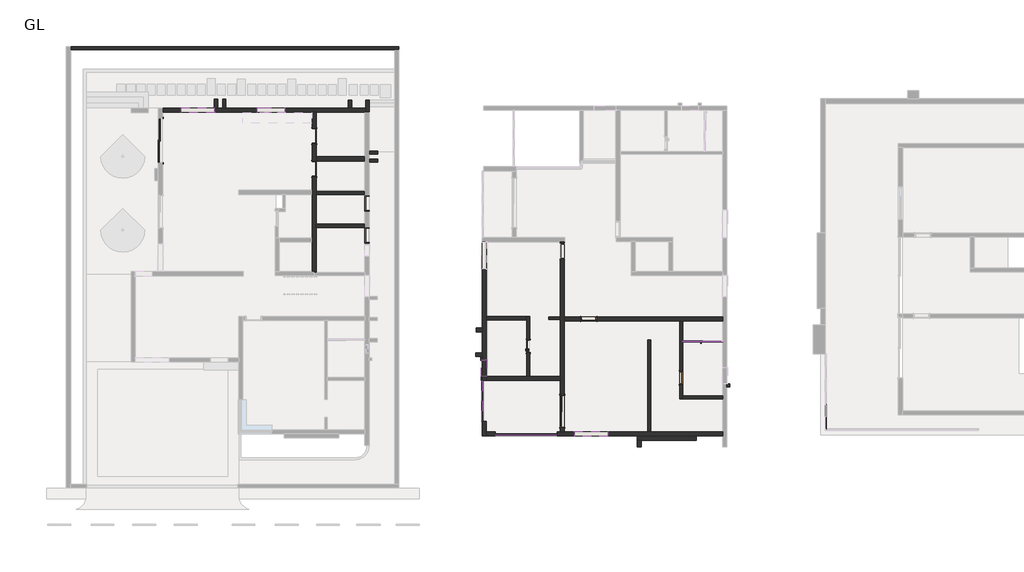
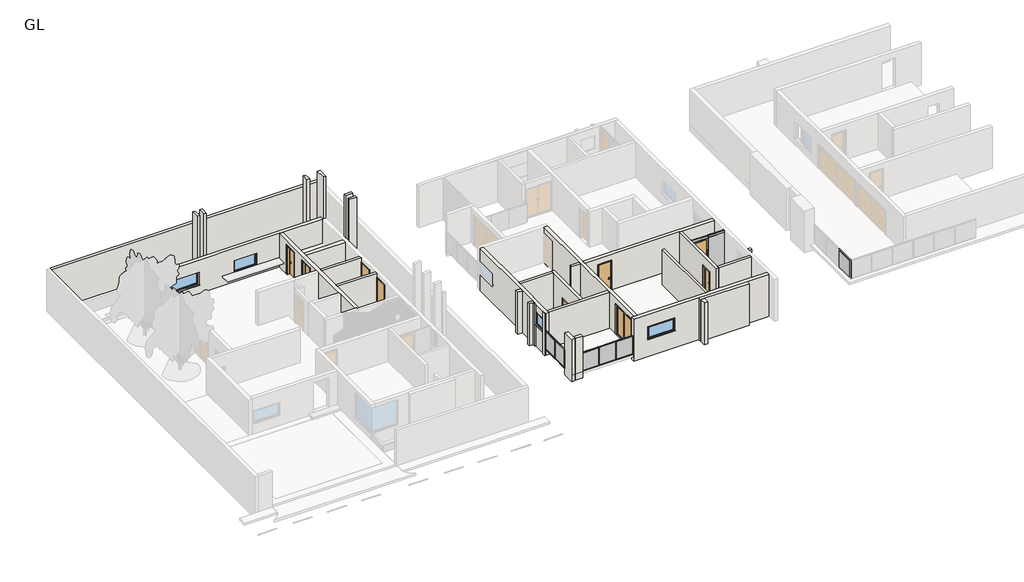
# One storey, part 2 of 6: 32 walls, 26 members, 10 doors, 9 plates, 4 windows.
"""IFC4 building model written with IfcOpenShell, lengths in millimetres."""

from ifc_helpers import new_model, si_unit, origin, origin_with_axes, place, context, project, spatial, polyline, outline, extrude, faceted_brep, transform, mapped, element, save
from components import door_510b0506, door_8_4088deed, door_61435f0d, door_b7cddb0a, doors_intsgl_2_5_55235da4, doors_intsgl_2_5_ea0f4f48, doors_sgl_glass_1_glass_panel_12mm_thickness_f5485519, rectangular_mullion_30mm_square_7ad516a4, rectangular_mullion_30mm_square_4b249e81, rectangular_mullion_30mm_square_698bad25, rectangular_mullion_30mm_square_c90eb03c, rectangular_mullion_30mm_square_82a776c0, rectangular_mullion_30mm_square_9325025b, rectangular_mullion_30mm_square_e994106c, rectangular_mullion_30mm_square_b4ecd99e, rectangular_mullion_30mm_square_28ebc8b3, rectangular_mullion_30mm_square_04db908b, rectangular_mullion_30mm_square_ca2d7245, system_panel_glazed_e1dbe616, system_panel_glazed_3d395eef, system_panel_glazed_b6747f4f, system_panel_glazed_7d86dfa2, system_panel_glazed_82719d7e, windows_sgl_plain_3_28d0678b, windows_sgl_plain_5_c2f68037, windows_sgl_plain_6_060cc830

model = new_model("IFC4")

# Units and contexts
model_context = context("Model", 3, world=origin())
ifc_project = project(units=[si_unit("LENGTHUNIT", "METRE", prefix="MILLI")], contexts=[model_context])

# Site, building, storey
site = spatial("IfcSite", under=ifc_project)
building = spatial("IfcBuilding", under=site)
storey = spatial("IfcBuildingStorey", under=building, Name="GL", Elevation=0.0)

# Doors
placement = place(None, origin())
door_shape = door_510b0506(model_context)
element("IfcDoor", 1, ObjectType="5'10\"", at=placement, inside=storey, context=model_context, shape_type="MappedRepresentation", body=[
    mapped(door_shape, transform((-24575.6081987, 10334.3302878, 449.9570313), x_axis=(0.0, 1.0, 0.0), y_axis=(-1.0, 0.0, 0.0), z_axis=(0.0, 0.0, 1.0))),
])
door_8_shape = door_8_4088deed(model_context)
element("IfcDoor", 2, ObjectType="8'", at=placement, inside=storey, context=model_context, shape_type="MappedRepresentation", body=[
    mapped(door_8_shape, transform((-46875.1786333, 25369.1148243, 449.9570313), x_axis=(0.0, 1.0, 0.0), y_axis=(-1.0, 0.0, 0.0), z_axis=(0.0, 0.0, 1.0))),
])
door_2_shape = door_61435f0d(model_context)
element("IfcDoor", 3, ObjectType="Doors_IntSgl : 2'11\"", at=placement, inside=storey, context=model_context, shape_type="MappedRepresentation", body=[
    mapped(door_2_shape, transform((-35537.04796, 20098.7041063, 589.9546875), x_axis=(0.0, 1.0, 0.0), y_axis=(-1.0, 0.0, 0.0), z_axis=(0.0, 0.0, 1.0))),
])
element("IfcDoor", 4, ObjectType="Doors_IntSgl : 2'11\"", at=placement, inside=storey, context=model_context, shape_type="MappedRepresentation", body=[
    mapped(door_2_shape, transform((-38458.04796, 25623.2041063, 589.9546875), x_axis=(0.0, -1.0, 0.0), y_axis=(1.0, 0.0, 0.0), z_axis=(0.0, 0.0, 1.0))),
])
element("IfcDoor", 5, ObjectType="Doors_IntSgl : 2'11\"", at=placement, inside=storey, context=model_context, shape_type="MappedRepresentation", body=[
    mapped(door_2_shape, transform((-35537.04796, 21876.7041063, 589.9546875), x_axis=(0.0, 1.0, 0.0), y_axis=(-1.0, 0.0, 0.0), z_axis=(0.0, 0.0, 1.0))),
])
element("IfcDoor", 6, ObjectType="Doors_IntSgl : 2'11\"", at=placement, inside=storey, context=model_context, shape_type="MappedRepresentation", body=[
    mapped(door_2_shape, transform((-23229.4081987, 15463.5822323, 449.9429688), x_axis=(-1.0, 0.0, 0.0), y_axis=(0.0, -1.0, 0.0), z_axis=(0.0, 0.0, 1.0))),
])
door_3_shape = door_b7cddb0a(model_context)
element("IfcDoor", 7, ObjectType="Doors_IntSgl : 2'11\"", at=placement, inside=storey, context=model_context, shape_type="MappedRepresentation", body=[
    mapped(door_3_shape, transform((-38458.04796, 23794.4041063, 589.9546875), x_axis=(0.0, 1.0, 0.0), y_axis=(-1.0, 0.0, 0.0), z_axis=(0.0, 0.0, 1.0))),
])
doors_intsgl_2_5_shape = doors_intsgl_2_5_55235da4(model_context)
element("IfcDoor", 8, ObjectType="Doors_IntSgl : 2.5'", at=placement, inside=storey, context=model_context, shape_type="MappedRepresentation", body=[
    mapped(doors_intsgl_2_5_shape, transform((-18095.11552, 12186.9822323, 449.9570313), x_axis=(0.0, 1.0, 0.0), y_axis=(-1.0, 0.0, 0.0), z_axis=(0.0, 0.0, 1.0))),
])
doors_intsgl_2_5_2_shape = doors_intsgl_2_5_ea0f4f48(model_context)
element("IfcDoor", 9, ObjectType="Doors_IntSgl : 2.5'", at=placement, inside=storey, context=model_context, shape_type="MappedRepresentation", body=[
    mapped(doors_intsgl_2_5_2_shape, transform((-26580.8290616, 13941.6413647, 0.0), x_axis=(0.0, 1.0, 0.0), y_axis=(-1.0, 0.0, 0.0), z_axis=(0.0, 0.0, 1.0))),
])
doors_sgl_glass_1_glass_panel_12mm_thickness_shape = doors_sgl_glass_1_glass_panel_12mm_thickness_f5485519(model_context)
element("IfcDoor", 10, ObjectType="Doors_Sgl_Glass_1 : Glass_Panel-12mm_Thickness", at=placement, inside=storey, context=model_context, shape_type="MappedRepresentation", body=[
    mapped(doors_sgl_glass_1_glass_panel_12mm_thickness_shape, transform((-17454.600712, 14231.6822323, 479.9570313), x_axis=(-1.0, 0.0, 0.0), y_axis=(0.0, -1.0, 0.0), z_axis=(0.0, 0.0, 1.0))),
])

# Members
rectangular_mullion_30mm_square_shape = rectangular_mullion_30mm_square_7ad516a4(model_context)
element("IfcMember", 11, ObjectType="Rectangular Mullion : 30mm_Square", at=placement, inside=storey, context=model_context, shape_type="MappedRepresentation", body=[
    mapped(rectangular_mullion_30mm_square_shape, transform((-29151.3790532, 10905.8302878, 449.9570313), x_axis=(0.0, -1.0, 0.0), y_axis=(-1.0, 0.0, 0.0), z_axis=(0.0, 0.0, -1.0))),
])
element("IfcMember", 12, ObjectType="Rectangular Mullion : 30mm_Square", at=placement, inside=storey, context=model_context, shape_type="MappedRepresentation", body=[
    mapped(rectangular_mullion_30mm_square_shape, transform((-27269.6623864, 9013.5302878, 449.9570313), x_axis=(1.0, 0.0, 0.0), y_axis=(0.0, -1.0, 0.0), z_axis=(0.0, 0.0, -1.0))),
])
element("IfcMember", 13, ObjectType="Rectangular Mullion : 30mm_Square", at=placement, inside=storey, context=model_context, shape_type="MappedRepresentation", body=[
    mapped(rectangular_mullion_30mm_square_shape, transform((-26118.19572, 9013.5302878, 449.9570313), x_axis=(1.0, 0.0, 0.0), y_axis=(0.0, -1.0, 0.0), z_axis=(0.0, 0.0, -1.0))),
])
rectangular_mullion_30mm_square_2_shape = rectangular_mullion_30mm_square_4b249e81(model_context)
element("IfcMember", 14, ObjectType="Rectangular Mullion : 30mm_Square", at=placement, inside=storey, context=model_context, shape_type="MappedRepresentation", body=[
    mapped(rectangular_mullion_30mm_square_2_shape, transform((-29151.3790532, 12036.1302878, 1780.8), x_axis=(0.0, 1.0, 0.0), y_axis=(-1.0, 0.0, 0.0), z_axis=(0.0, 0.0, 1.0))),
])
element("IfcMember", 15, ObjectType="Rectangular Mullion : 30mm_Square", at=placement, inside=storey, context=model_context, shape_type="MappedRepresentation", body=[
    mapped(rectangular_mullion_30mm_square_2_shape, transform((-28421.1290532, 9013.5302878, 1780.8), x_axis=(-1.0, 0.0, 0.0), y_axis=(0.0, -1.0, 0.0), z_axis=(0.0, 0.0, 1.0))),
])
element("IfcMember", 16, ObjectType="Rectangular Mullion : 30mm_Square", at=placement, inside=storey, context=model_context, shape_type="MappedRepresentation", body=[
    mapped(rectangular_mullion_30mm_square_2_shape, transform((-29151.3790532, 9775.5302878, 449.9570313), x_axis=(0.0, -1.0, 0.0), y_axis=(-1.0, 0.0, 0.0), z_axis=(0.0, 0.0, -1.0))),
])
element("IfcMember", 17, ObjectType="Rectangular Mullion : 30mm_Square", at=placement, inside=storey, context=model_context, shape_type="MappedRepresentation", body=[
    mapped(rectangular_mullion_30mm_square_2_shape, transform((-24966.7290532, 9013.5302878, 449.9570313), x_axis=(1.0, 0.0, 0.0), y_axis=(0.0, -1.0, 0.0), z_axis=(0.0, 0.0, -1.0))),
])
rectangular_mullion_30mm_square_3_shape = rectangular_mullion_30mm_square_698bad25(model_context)
element("IfcMember", 18, ObjectType="Rectangular Mullion : 30mm_Square", at=placement, inside=storey, context=model_context, shape_type="MappedRepresentation", body=[
    mapped(rectangular_mullion_30mm_square_3_shape, transform((-29151.3790532, 9805.5302878, 1780.8), x_axis=(0.0, 0.0, 1.0), y_axis=(-1.0, 0.0, 0.0), z_axis=(0.0, -1.0, 0.0))),
])
element("IfcMember", 19, ObjectType="Rectangular Mullion : 30mm_Square", at=placement, inside=storey, context=model_context, shape_type="MappedRepresentation", body=[
    mapped(rectangular_mullion_30mm_square_3_shape, transform((-29151.3790532, 10920.8302878, 1780.8), x_axis=(0.0, 0.0, 1.0), y_axis=(-1.0, 0.0, 0.0), z_axis=(0.0, -1.0, 0.0))),
])
element("IfcMember", 20, ObjectType="Rectangular Mullion : 30mm_Square", at=placement, inside=storey, context=model_context, shape_type="MappedRepresentation", body=[
    mapped(rectangular_mullion_30mm_square_3_shape, transform((-29151.3790532, 12006.1302878, 449.9570313), x_axis=(0.0, 0.0, -1.0), y_axis=(-1.0, 0.0, 0.0), z_axis=(0.0, 1.0, 0.0))),
])
element("IfcMember", 21, ObjectType="Rectangular Mullion : 30mm_Square", at=placement, inside=storey, context=model_context, shape_type="MappedRepresentation", body=[
    mapped(rectangular_mullion_30mm_square_3_shape, transform((-29151.3790532, 10890.8302878, 449.9570313), x_axis=(0.0, 0.0, -1.0), y_axis=(-1.0, 0.0, 0.0), z_axis=(0.0, 1.0, 0.0))),
])
rectangular_mullion_30mm_square_4_shape = rectangular_mullion_30mm_square_c90eb03c(model_context)
element("IfcMember", 22, ObjectType="Rectangular Mullion : 30mm_Square", at=placement, inside=storey, context=model_context, shape_type="MappedRepresentation", body=[
    mapped(rectangular_mullion_30mm_square_4_shape, transform((-24996.7290532, 9013.5302878, 1780.8), x_axis=(0.0, 0.0, 1.0), y_axis=(0.0, -1.0, 0.0), z_axis=(1.0, 0.0, 0.0))),
])
element("IfcMember", 23, ObjectType="Rectangular Mullion : 30mm_Square", at=placement, inside=storey, context=model_context, shape_type="MappedRepresentation", body=[
    mapped(rectangular_mullion_30mm_square_4_shape, transform((-27284.6623864, 9013.5302878, 1780.8), x_axis=(0.0, 0.0, 1.0), y_axis=(0.0, -1.0, 0.0), z_axis=(1.0, 0.0, 0.0))),
])
element("IfcMember", 24, ObjectType="Rectangular Mullion : 30mm_Square", at=placement, inside=storey, context=model_context, shape_type="MappedRepresentation", body=[
    mapped(rectangular_mullion_30mm_square_4_shape, transform((-28391.1290532, 9013.5302878, 449.9570313), x_axis=(0.0, 0.0, -1.0), y_axis=(0.0, -1.0, 0.0), z_axis=(-1.0, 0.0, 0.0))),
])
element("IfcMember", 25, ObjectType="Rectangular Mullion : 30mm_Square", at=placement, inside=storey, context=model_context, shape_type="MappedRepresentation", body=[
    mapped(rectangular_mullion_30mm_square_4_shape, transform((-26103.19572, 9013.5302878, 449.9570313), x_axis=(0.0, 0.0, -1.0), y_axis=(0.0, -1.0, 0.0), z_axis=(-1.0, 0.0, 0.0))),
])
rectangular_mullion_30mm_square_5_shape = rectangular_mullion_30mm_square_82a776c0(model_context)
element("IfcMember", 26, ObjectType="Rectangular Mullion : 30mm_Square", at=placement, inside=storey, context=model_context, shape_type="MappedRepresentation", body=[
    mapped(rectangular_mullion_30mm_square_5_shape, transform((-27254.6623864, 9013.5302878, 449.9570313), x_axis=(0.0, 0.0, -1.0), y_axis=(0.0, -1.0, 0.0), z_axis=(-1.0, 0.0, 0.0))),
])
element("IfcMember", 27, ObjectType="Rectangular Mullion : 30mm_Square", at=placement, inside=storey, context=model_context, shape_type="MappedRepresentation", body=[
    mapped(rectangular_mullion_30mm_square_5_shape, transform((-26133.19572, 9013.5302878, 1780.8), x_axis=(0.0, 0.0, 1.0), y_axis=(0.0, -1.0, 0.0), z_axis=(1.0, 0.0, 0.0))),
])
rectangular_mullion_30mm_square_6_shape = rectangular_mullion_30mm_square_9325025b(model_context)
element("IfcMember", 28, ObjectType="Rectangular Mullion : 30mm_Square", at=placement, inside=storey, context=model_context, shape_type="MappedRepresentation", body=[
    mapped(rectangular_mullion_30mm_square_6_shape, transform((-16905.2859039, 14231.6822323, 449.9570313), x_axis=(-1.0, 0.0, 0.0), y_axis=(0.0, 1.0, 0.0), z_axis=(0.0, 0.0, -1.0))),
])
rectangular_mullion_30mm_square_7_shape = rectangular_mullion_30mm_square_e994106c(model_context)
element("IfcMember", 29, ObjectType="Rectangular Mullion : 30mm_Square", at=placement, inside=storey, context=model_context, shape_type="MappedRepresentation", body=[
    mapped(rectangular_mullion_30mm_square_7_shape, transform((-16905.2859039, 14231.6822323, 2849.9570312), x_axis=(-1.0, 0.0, 0.0), y_axis=(0.0, 1.0, 0.0), z_axis=(0.0, 0.0, -1.0))),
])
rectangular_mullion_30mm_square_8_shape = rectangular_mullion_30mm_square_b4ecd99e(model_context)
element("IfcMember", 30, ObjectType="Rectangular Mullion : 30mm_Square", at=placement, inside=storey, context=model_context, shape_type="MappedRepresentation", body=[
    mapped(rectangular_mullion_30mm_square_8_shape, transform((-18018.91552, 14231.6822323, 449.9570313), x_axis=(-1.0, 0.0, 0.0), y_axis=(0.0, 1.0, 0.0), z_axis=(0.0, 0.0, -1.0))),
])
rectangular_mullion_30mm_square_9_shape = rectangular_mullion_30mm_square_28ebc8b3(model_context)
element("IfcMember", 31, ObjectType="Rectangular Mullion : 30mm_Square", at=placement, inside=storey, context=model_context, shape_type="MappedRepresentation", body=[
    mapped(rectangular_mullion_30mm_square_9_shape, transform((-18018.91552, 14231.6822323, 2849.9570312), x_axis=(-1.0, 0.0, 0.0), y_axis=(0.0, 1.0, 0.0), z_axis=(0.0, 0.0, -1.0))),
])
rectangular_mullion_30mm_square_10_shape = rectangular_mullion_30mm_square_04db908b(model_context)
element("IfcMember", 32, ObjectType="Rectangular Mullion : 30mm_Square", at=placement, inside=storey, context=model_context, shape_type="MappedRepresentation", body=[
    mapped(rectangular_mullion_30mm_square_10_shape, transform((-17988.91552, 14231.6822323, 3000.0), x_axis=(0.0, 0.0, 1.0), y_axis=(0.0, 1.0, 0.0), z_axis=(-1.0, 0.0, 0.0))),
])
element("IfcMember", 33, ObjectType="Rectangular Mullion : 30mm_Square", at=placement, inside=storey, context=model_context, shape_type="MappedRepresentation", body=[
    mapped(rectangular_mullion_30mm_square_10_shape, transform((-16890.2859039, 14231.6822323, 3000.0), x_axis=(0.0, 0.0, 1.0), y_axis=(0.0, 1.0, 0.0), z_axis=(-1.0, 0.0, 0.0))),
])
element("IfcMember", 34, ObjectType="Rectangular Mullion : 30mm_Square", at=placement, inside=storey, context=model_context, shape_type="MappedRepresentation", body=[
    mapped(rectangular_mullion_30mm_square_10_shape, transform((-16920.2859039, 14231.6822323, 449.9570313), x_axis=(0.0, 0.0, -1.0), y_axis=(0.0, 1.0, 0.0), z_axis=(1.0, 0.0, 0.0))),
])
rectangular_mullion_30mm_square_11_shape = rectangular_mullion_30mm_square_ca2d7245(model_context)
element("IfcMember", 35, ObjectType="Rectangular Mullion : 30mm_Square", at=placement, inside=storey, context=model_context, shape_type="MappedRepresentation", body=[
    mapped(rectangular_mullion_30mm_square_11_shape, transform((-16890.2859039, 14231.6822323, 2849.9570312), x_axis=(0.0, 0.0, 1.0), y_axis=(0.0, 1.0, 0.0), z_axis=(-1.0, 0.0, 0.0))),
])
element("IfcMember", 36, ObjectType="Rectangular Mullion : 30mm_Square", at=placement, inside=storey, context=model_context, shape_type="MappedRepresentation", body=[
    mapped(rectangular_mullion_30mm_square_11_shape, transform((-17988.91552, 14231.6822323, 2849.9570312), x_axis=(0.0, 0.0, 1.0), y_axis=(0.0, 1.0, 0.0), z_axis=(-1.0, 0.0, 0.0))),
])

# Plates
system_panel_glazed_shape = system_panel_glazed_e1dbe616(model_context)
element("IfcPlate", 37, ObjectType="System Panel : Glazed", at=placement, inside=storey, context=model_context, shape_type="MappedRepresentation", body=[
    mapped(system_panel_glazed_shape, transform((-29151.3790532, 11470.9802878, 449.9570313), x_axis=(0.0, -1.0, 0.0), y_axis=(1.0, 0.0, 0.0), z_axis=(0.0, 0.0, 1.0))),
])
element("IfcPlate", 38, ObjectType="System Panel : Glazed", at=placement, inside=storey, context=model_context, shape_type="MappedRepresentation", body=[
    mapped(system_panel_glazed_shape, transform((-29151.3790532, 10340.6802878, 449.9570313), x_axis=(0.0, -1.0, 0.0), y_axis=(1.0, 0.0, 0.0), z_axis=(0.0, 0.0, 1.0))),
])
system_panel_glazed_2_shape = system_panel_glazed_3d395eef(model_context)
element("IfcPlate", 39, ObjectType="System Panel : Glazed", at=placement, inside=storey, context=model_context, shape_type="MappedRepresentation", body=[
    mapped(system_panel_glazed_2_shape, transform((-27845.3957198, 9013.5302878, 449.9570313), x_axis=(1.0, 0.0, 0.0), y_axis=(0.0, 1.0, 0.0), z_axis=(0.0, 0.0, 1.0))),
])
element("IfcPlate", 40, ObjectType="System Panel : Glazed", at=placement, inside=storey, context=model_context, shape_type="MappedRepresentation", body=[
    mapped(system_panel_glazed_2_shape, transform((-26693.9290532, 9013.5302878, 449.9570313), x_axis=(1.0, 0.0, 0.0), y_axis=(0.0, 1.0, 0.0), z_axis=(0.0, 0.0, 1.0))),
])
element("IfcPlate", 41, ObjectType="System Panel : Glazed", at=placement, inside=storey, context=model_context, shape_type="MappedRepresentation", body=[
    mapped(system_panel_glazed_2_shape, transform((-25542.4623866, 9013.5302878, 449.9570313), x_axis=(1.0, 0.0, 0.0), y_axis=(0.0, 1.0, 0.0), z_axis=(0.0, 0.0, 1.0))),
])
system_panel_glazed_3_shape = system_panel_glazed_b6747f4f(model_context)
element("IfcPlate", 42, ObjectType="System Panel : Glazed", at=placement, inside=storey, context=model_context, shape_type="MappedRepresentation", body=[
    mapped(system_panel_glazed_3_shape, transform((-10088.6061453, 9998.7340034, 449.9570313), x_axis=(0.0, -1.0, 0.0), y_axis=(1.0, 0.0, 0.0), z_axis=(0.0, 0.0, 1.0))),
])
system_panel_glazed_4_shape = system_panel_glazed_7d86dfa2(model_context)
element("IfcPlate", 43, ObjectType="System Panel : Glazed", at=placement, inside=storey, context=model_context, shape_type="MappedRepresentation", body=[
    mapped(system_panel_glazed_4_shape, transform((-16348.4710959, 14231.6822323, 449.9570313), x_axis=(-1.0, 0.0, 0.0), y_axis=(0.0, -1.0, 0.0), z_axis=(0.0, 0.0, 1.0))),
])
system_panel_glazed_5_shape = system_panel_glazed_82719d7e(model_context)
element("IfcPlate", 44, ObjectType="System Panel : Glazed", at=placement, inside=storey, context=model_context, shape_type="MappedRepresentation", body=[
    mapped(system_panel_glazed_5_shape, transform((-16348.4710959, 14231.6822323, 2849.9570312), x_axis=(-1.0, 0.0, 0.0), y_axis=(0.0, -1.0, 0.0), z_axis=(0.0, 0.0, 1.0))),
])
element("IfcPlate", 45, ObjectType="System Panel : Glazed", at=placement, inside=storey, context=model_context, shape_type="MappedRepresentation", body=[
    mapped(system_panel_glazed_5_shape, transform((-17462.100712, 14231.6822323, 2849.9570312), x_axis=(-1.0, 0.0, 0.0), y_axis=(0.0, -1.0, 0.0), z_axis=(0.0, 0.0, 1.0))),
])

# Walls
element("IfcWall", 46, ObjectType="6\" WALL", at=placement, inside=storey, context=model_context, shape_type="SweptSolid", body=[
    extrude(outline(polyline([(-35422.74796, 24337.1254786), (-34938.0119863, 24337.1254786), (-34938.0119863, 24184.7254786), (-35422.74796, 24184.7254786), (-35422.74796, 24337.1254786)])), origin_with_axes(), (0.0, 0.0, 1.0), 6000.0),
])
element("IfcWall", 47, ObjectType="6\" WALL", at=placement, inside=storey, context=model_context, shape_type="SweptSolid", body=[
    extrude(outline(polyline([(-25439.2081987, 15577.8822323), (-24816.9081987, 15577.8822323), (-24816.9081987, 15425.4822323), (-25439.2081987, 15425.4822323), (-25439.2081987, 15577.8822323)])), origin_with_axes(), (0.0, 0.0, 1.0), 3000.0),
])
element("IfcWall", 48, ObjectType="6\" WALL", at=placement, inside=storey, context=model_context, shape_type="SweptSolid", body=[
    extrude(outline(polyline([(-19796.5546362, 14284.0302878), (-19796.5546362, 9191.3302878), (-19948.9546362, 9191.3302878), (-19948.9546362, 14284.0302878), (-19796.5546362, 14284.0302878)])), origin_with_axes(), (0.0, 0.0, 1.0), 3000.0),
])
element("IfcWall", 49, ObjectType="6\" WALL", at=placement, inside=storey, context=model_context, shape_type="Brep", body=[
    faceted_brep([(-18171.31552, 15349.2822323, 0.0), (-18171.31552, 11018.5822323, 0.0), (-18171.31552, 11018.5822323, 3000.0), (-18171.31552, 15349.2822323, 3000.0), (-18171.31552, 12567.9822323, 449.9570313), (-18171.31552, 12567.9822323, 2278.7570313), (-18171.31552, 11805.9822323, 2278.7570313), (-18171.31552, 11805.9822323, 449.9570313), (-18018.91552, 11018.5822323, 0.0), (-18018.91552, 11196.3822323, 0.0), (-18018.91552, 15349.2822323, 0.0), (-18018.91552, 15349.2822323, 3000.0), (-18018.91552, 11196.3822323, 3000.0), (-18018.91552, 11018.5822323, 3000.0), (-18018.91552, 12567.9822323, 2278.7570313), (-18018.91552, 12567.9822323, 449.9570313), (-18018.91552, 11805.9822323, 449.9570313), (-18018.91552, 11805.9822323, 2278.7570312)], [[[0, 1, 2, 3], [4, 5, 6, 7]], [[8, 9, 10, 11, 12, 13], [14, 15, 16, 17]], [[1, 0, 10, 9, 8]], [[3, 2, 13, 12, 11]], [[0, 3, 11, 10]], [[2, 1, 8, 13]], [[4, 15, 14, 5]], [[5, 14, 17, 6]], [[6, 17, 16, 7]], [[15, 4, 7, 16]]]),
])
element("IfcWall", 50, ObjectType="7\" WALL", at=placement, inside=storey, context=model_context, shape_type="SweptSolid", body=[
    extrude(outline(polyline([(-38343.74796, 20721.0041063), (-35651.34796, 20721.0041063), (-35651.34796, 20543.2041063), (-38343.74796, 20543.2041063), (-38343.74796, 20721.0041063)])), origin_with_axes(), (0.0, 0.0, 1.0), 3000.0),
])
element("IfcWall", 51, ObjectType="7\" WALL", at=placement, inside=storey, context=model_context, shape_type="SweptSolid", body=[
    extrude(outline(polyline([(-38343.74796, 22549.8041063), (-35651.34796, 22549.8041063), (-35651.34796, 22372.0041063), (-38343.74796, 22372.0041063), (-38343.74796, 22549.8041063)])), origin_with_axes(), (0.0, 0.0, 1.0), 3000.0),
])
element("IfcWall", 52, ObjectType="7\" WALL", at=placement, inside=storey, context=model_context, shape_type="Brep", body=[
    faceted_brep([(-51999.5791975, 30421.4065956, 0.0), (-33990.9791975, 30421.4065956, 0.0), (-33762.3791975, 30421.4065956, 0.0), (-33762.3791975, 30421.4065956, 3000.0), (-33990.9791975, 30421.4065956, 3000.0), (-51999.5791975, 30421.4065956, 3000.0), (-51999.5791975, 30599.2065956, 0.0), (-51999.5791975, 30599.2065956, 3000.0), (-33762.3791975, 30599.2065956, 3000.0), (-33762.3791975, 30599.2065956, 0.0)], [[[0, 1, 2, 3, 4, 5]], [[6, 7, 8, 9]], [[2, 1, 0, 6, 9]], [[5, 4, 3, 8, 7]], [[0, 5, 7, 6]], [[3, 2, 9, 8]]]),
])
element("IfcWall", 53, ObjectType="7\" WALL", at=placement, inside=storey, context=model_context, shape_type="SweptSolid", body=[
    extrude(outline(polyline([(-44010.1992487, 27172.5148243), (-44010.1992487, 27671.0783647), (-43832.3992487, 27671.0783647), (-43832.3992487, 27172.5148243), (-44010.1992487, 27172.5148243)])), origin_with_axes(), (0.0, 0.0, 1.0), 6000.0),
])
element("IfcWall", 54, ObjectType="7\" WALL", at=placement, inside=storey, context=model_context, shape_type="SweptSolid", body=[
    extrude(outline(polyline([(-43552.9992487, 27172.5148243), (-43552.9992487, 27671.0783647), (-43375.1992487, 27671.0783647), (-43375.1992487, 27172.5148243), (-43552.9992487, 27172.5148243)])), origin_with_axes(), (0.0, 0.0, 1.0), 6000.0),
])
element("IfcWall", 55, ObjectType="7\" WALL", at=placement, inside=storey, context=model_context, shape_type="SweptSolid", body=[
    extrude(outline(polyline([(-36568.3688545, 27172.5148243), (-36568.3688545, 27628.0855094), (-36390.5688545, 27628.0855094), (-36390.5688545, 27172.5148243), (-36568.3688545, 27172.5148243)])), origin_with_axes(), (0.0, 0.0, 1.0), 6000.0),
])
element("IfcWall", 56, ObjectType="7\" WALL", at=placement, inside=storey, context=model_context, shape_type="Brep", body=[
    faceted_brep([(-35600.54796, 27628.0855094, 0.0), (-35600.54796, 27172.5148243, 0.0), (-35600.54796, 26943.9148243, 0.0), (-35600.54796, 26943.9148243, 3000.0), (-35600.54796, 26943.9148243, 6000.0), (-35600.54796, 27628.0855094, 6000.0), (-35422.74796, 27628.0855094, 0.0), (-35422.74796, 27628.0855094, 6000.0), (-35422.74796, 26943.9148243, 6000.0), (-35422.74796, 26943.9148243, 3000.0), (-35422.74796, 26943.9148243, 0.0)], [[[0, 1, 2, 3, 4, 5]], [[6, 7, 8, 9, 10]], [[2, 1, 0, 6, 10]], [[5, 4, 8, 7]], [[0, 5, 7, 6]], [[4, 3, 2, 10, 9, 8]]]),
])
element("IfcWall", 57, ObjectType="7\" WALL", at=placement, inside=storey, context=model_context, shape_type="SweptSolid", body=[
    extrude(outline(polyline([(-35422.74796, 24797.7041063), (-34938.0119863, 24797.7041063), (-34938.0119863, 24619.9041063), (-35422.74796, 24619.9041063), (-35422.74796, 24797.7041063)])), origin_with_axes(), (0.0, 0.0, 1.0), 6000.0),
])
element("IfcWall", 58, ObjectType="7\" WALL", at=placement, inside=storey, context=model_context, shape_type="Brep", body=[
    faceted_brep([(-26491.9290616, 15592.6413647, 3000.0), (-26491.9290616, 12265.2413647, 3000.0), (-26491.9290616, 12265.2413647, 0.0), (-26491.9290616, 13560.6413647, 0.0), (-26491.9290616, 13560.6413647, 1828.8), (-26491.9290616, 14322.6413647, 1828.8), (-26491.9290616, 14322.6413647, 0.0), (-26491.9290616, 15592.6413647, 0.0), (-26669.7290616, 12265.2413647, 3000.0), (-26669.7290616, 15414.8413647, 3000.0), (-26669.7290616, 15592.6413647, 3000.0), (-26669.7290616, 15592.6413647, 0.0), (-26669.7290616, 15414.8413647, 0.0), (-26669.7290616, 14322.6413647, 0.0), (-26669.7290616, 14322.6413647, 1828.8), (-26669.7290616, 13560.6413647, 1828.8), (-26669.7290616, 13560.6413647, 0.0), (-26669.7290616, 12265.2413647, 0.0)], [[[0, 1, 2, 3, 4, 5, 6, 7]], [[8, 9, 10, 11, 12, 13, 14, 15, 16, 17]], [[2, 17, 16, 3]], [[11, 7, 6, 13, 12]], [[1, 0, 10, 9, 8]], [[2, 1, 8, 17]], [[0, 7, 11, 10]], [[5, 14, 13, 6]], [[14, 5, 4, 15]], [[15, 4, 3, 16]]]),
])
element("IfcWall", 59, ObjectType="7\" WALL", at=placement, inside=storey, context=model_context, shape_type="SweptSolid", body=[
    extrude(outline(polyline([(-28922.7790532, 15592.6413647), (-26669.7290616, 15592.6413647), (-26669.7290616, 15414.8413647), (-28922.7790532, 15414.8413647), (-28922.7790532, 15592.6413647)])), origin_with_axes(), (0.0, 0.0, 1.0), 3000.0),
])
element("IfcWall", 60, ObjectType="7\" WALL", at=placement, inside=storey, context=model_context, shape_type="SweptSolid", body=[
    extrude(outline(polyline([(-15785.4464918, 11018.5822323), (-18018.91552, 11018.5822323), (-18018.91552, 11196.3822323), (-15785.4464918, 11196.3822323), (-15785.4464918, 11018.5822323)])), origin_with_axes(), (0.0, 0.0, 1.0), 3000.0),
])
element("IfcWall", 61, ObjectType="7\" WALL", at=placement, inside=storey, context=model_context, shape_type="SweptSolid", body=[
    extrude(outline(polyline([(-15405.9016085, 11672.6322323), (-15556.8464918, 11672.6322323), (-15556.8464918, 11850.4322323), (-15405.9016085, 11850.4322323), (-15405.9016085, 11672.6322323)])), origin_with_axes(), (0.0, 0.0, 1.0), 3000.0),
])
element("IfcWall", 62, ObjectType="7\" WALL", at=placement, inside=storey, context=model_context, shape_type="SweptSolid", body=[
    extrude(outline(polyline([(-29487.9290532, 13564.0513246), (-29151.3790532, 13564.0513246), (-29151.3790532, 13386.2513246), (-29487.9290532, 13386.2513246), (-29487.9290532, 13564.0513246)])), origin_with_axes(), (0.0, 0.0, 1.0), 3000.0),
])
element("IfcWall", 63, ObjectType="9\" INNER WALL", at=placement, inside=storey, context=model_context, shape_type="Brep", body=[
    faceted_brep([(-46887.8786333, 26943.9148243, 0.0), (-38572.34796, 26943.9148243, 0.0), (-38343.74796, 26943.9148243, 0.0), (-35651.34796, 26943.9148243, 0.0), (-35600.54796, 26943.9148243, 0.0), (-35600.54796, 26943.9148243, 3000.0), (-35651.34796, 26943.9148243, 3000.0), (-38343.74796, 26943.9148243, 3000.0), (-38572.34796, 26943.9148243, 3000.0), (-46887.8786333, 26943.9148243, 3000.0), (-40096.34796, 26943.9148243, 2110.0), (-40096.34796, 26943.9148243, 1200.0), (-41620.34796, 26943.9148243, 1200.0), (-41620.34796, 26943.9148243, 2110.0), (-45838.9992487, 26943.9148243, 2110.0), (-44010.1992487, 26943.9148243, 2110.0), (-44010.1992487, 26943.9148243, 1200.0), (-45838.9992487, 26943.9148243, 1200.0), (-46887.8786333, 27172.5148243, 0.0), (-46887.8786333, 27172.5148243, 3000.0), (-35600.54796, 27172.5148243, 3000.0), (-35600.54796, 27172.5148243, 0.0), (-36390.5688545, 27172.5148243, 0.0), (-36568.3688545, 27172.5148243, 0.0), (-43375.1992487, 27172.5148243, 0.0), (-43552.9992487, 27172.5148243, 0.0), (-43832.3992487, 27172.5148243, 0.0), (-44010.1992487, 27172.5148243, 0.0), (-40096.34796, 27172.5148243, 2110.0), (-41620.34796, 27172.5148243, 2110.0), (-41620.34796, 27172.5148243, 1200.0), (-40096.34796, 27172.5148243, 1200.0), (-45838.9992487, 27172.5148243, 2110.0), (-45838.9992487, 27172.5148243, 1200.0), (-44010.1992487, 27172.5148243, 1200.0), (-44010.1992487, 27172.5148243, 2110.0)], [[[0, 1, 2, 3, 4, 5, 6, 7, 8, 9], [10, 11, 12, 13], [14, 15, 16, 17]], [[18, 19, 20, 21, 22, 23, 24, 25, 26, 27], [28, 29, 30, 31], [32, 33, 34, 35]], [[4, 3, 2, 1, 0, 18, 27, 26, 25, 24, 23, 22, 21]], [[9, 8, 7, 6, 5, 20, 19]], [[0, 9, 19, 18]], [[5, 4, 21, 20]], [[11, 10, 28, 31]], [[12, 11, 31, 30]], [[13, 12, 30, 29]], [[10, 13, 29, 28]], [[33, 32, 14, 17]], [[34, 33, 17, 16]], [[35, 34, 16, 15]], [[32, 35, 15, 14]]]),
])
element("IfcWall", 64, ObjectType="9\" INNER WALL", at=placement, inside=storey, context=model_context, shape_type="Brep", body=[
    faceted_brep([(-38343.74796, 18041.3041063, 0.0), (-38343.74796, 20543.2041063, 0.0), (-38343.74796, 20721.0041063, 0.0), (-38343.74796, 22372.0041063, 0.0), (-38343.74796, 22549.8041063, 0.0), (-38343.74796, 24238.9041063, 0.0), (-38343.74796, 24492.9041063, 0.0), (-38343.74796, 26943.9148243, 0.0), (-38343.74796, 26943.9148243, 3000.0), (-38343.74796, 24492.9041063, 3000.0), (-38343.74796, 24238.9041063, 3000.0), (-38343.74796, 22549.8041063, 3000.0), (-38343.74796, 22372.0041063, 3000.0), (-38343.74796, 20721.0041063, 3000.0), (-38343.74796, 20543.2041063, 3000.0), (-38343.74796, 18041.3041063, 3000.0), (-38343.74796, 25178.7041063, 589.9546875), (-38343.74796, 25178.7041063, 2699.9546875), (-38343.74796, 26067.7041063, 2699.9546875), (-38343.74796, 26067.7041063, 589.9546875), (-38343.74796, 24238.9041063, 2699.9546875), (-38343.74796, 24238.9041063, 589.9546875), (-38343.74796, 23349.9041063, 589.9546875), (-38343.74796, 23349.9041063, 2699.9546875), (-38572.34796, 26943.9148243, 0.0), (-38572.34796, 22613.3041063, 0.0), (-38572.34796, 22359.3041063, 0.0), (-38572.34796, 19959.0041063, 0.0), (-38572.34796, 19730.4041063, 0.0), (-38572.34796, 18092.1041063, 0.0), (-38572.34796, 18092.1041063, 3000.0), (-38572.34796, 19730.4041063, 3000.0), (-38572.34796, 19959.0041063, 3000.0), (-38572.34796, 22359.3041063, 3000.0), (-38572.34796, 22613.3041063, 3000.0), (-38572.34796, 26943.9148243, 3000.0), (-38572.34796, 25178.7041063, 2699.9546875), (-38572.34796, 25178.7041063, 589.9546875), (-38572.34796, 26067.7041063, 589.9546875), (-38572.34796, 26067.7041063, 2699.9546875), (-38572.34796, 24238.9041063, 589.9546875), (-38572.34796, 24238.9041063, 2699.9546875), (-38572.34796, 23349.9041063, 2699.9546875), (-38572.34796, 23349.9041063, 589.9546875), (-38458.04796, 18041.3041063, 0.0), (-38458.04796, 18092.1041063, 0.0), (-38458.04796, 18092.1041063, 3000.0), (-38458.04796, 18041.3041063, 3000.0)], [[[0, 1, 2, 3, 4, 5, 6, 7, 8, 9, 10, 11, 12, 13, 14, 15], [16, 17, 18, 19], [20, 21, 22, 23]], [[24, 25, 26, 27, 28, 29, 30, 31, 32, 33, 34, 35], [36, 37, 38, 39], [40, 41, 42, 43]], [[7, 6, 5, 4, 3, 2, 1, 0, 44, 45, 29, 28, 27, 26, 25, 24]], [[15, 14, 13, 12, 11, 10, 9, 8, 35, 34, 33, 32, 31, 30, 46, 47]], [[0, 15, 47, 44]], [[47, 46, 45, 44]], [[30, 29, 45, 46]], [[8, 7, 24, 35]], [[16, 37, 36, 17]], [[17, 36, 39, 18]], [[18, 39, 38, 19]], [[37, 16, 19, 38]], [[40, 21, 20, 41]], [[41, 20, 23, 42]], [[22, 43, 42, 23]], [[21, 40, 43, 22]]]),
])
element("IfcWall", 65, ObjectType="9\" INNER WALL", at=placement, inside=storey, context=model_context, shape_type="Brep", body=[
    faceted_brep([(-29151.3790532, 19746.9424071, 3000.0), (-29151.3790532, 19746.9424071, 2110.0), (-29151.3790532, 18222.9424071, 2110.0), (-29151.3790532, 18222.9424071, 1200.0), (-29151.3790532, 19746.9424071, 1200.0), (-29151.3790532, 19746.9424071, 0.0), (-29151.3790532, 14957.6413647, 0.0), (-29151.3790532, 14729.0413647, 0.0), (-29151.3790532, 13564.0513246, 0.0), (-29151.3790532, 13386.2513246, 0.0), (-29151.3790532, 13157.6513246, 0.0), (-29151.3790532, 12277.9413647, 0.0), (-29151.3790532, 12049.3413647, 0.0), (-29151.3790532, 12036.1302878, 0.0), (-29151.3790532, 12036.1302878, 3000.0), (-29151.3790532, 12049.3413647, 3000.0), (-29151.3790532, 12277.9413647, 3000.0), (-29151.3790532, 13157.6513246, 3000.0), (-29151.3790532, 13386.2513246, 3000.0), (-29151.3790532, 13564.0513246, 3000.0), (-29151.3790532, 14729.0413647, 3000.0), (-29151.3790532, 14957.6413647, 3000.0), (-29151.3790532, 12277.9413647, 2434.0), (-29151.3790532, 12277.9413647, 1524.0), (-29151.3790532, 13192.3413647, 1524.0), (-29151.3790532, 13192.3413647, 2434.0), (-28922.7790532, 18222.9424071, 2110.0), (-28922.7790532, 19746.9424071, 2110.0), (-28922.7790532, 19746.9424071, 3000.0), (-28922.7790532, 15592.6413647, 3000.0), (-28922.7790532, 15414.8413647, 3000.0), (-28922.7790532, 12265.2413647, 3000.0), (-28922.7790532, 12036.6413647, 3000.0), (-28922.7790532, 12036.1302878, 3000.0), (-28922.7790532, 12036.1302878, 0.0), (-28922.7790532, 12036.6413647, 0.0), (-28922.7790532, 12265.2413647, 0.0), (-28922.7790532, 15414.8413647, 0.0), (-28922.7790532, 15592.6413647, 0.0), (-28922.7790532, 19746.9424071, 0.0), (-28922.7790532, 19746.9424071, 1200.0), (-28922.7790532, 18222.9424071, 1200.0), (-28922.7790532, 12277.9413647, 2434.0), (-28922.7790532, 13192.3413647, 2434.0), (-28922.7790532, 13192.3413647, 1524.0), (-28922.7790532, 12277.9413647, 1524.0)], [[[0, 1, 2, 3, 4, 5, 6, 7, 8, 9, 10, 11, 12, 13, 14, 15, 16, 17, 18, 19, 20, 21], [22, 23, 24, 25]], [[26, 27, 28, 29, 30, 31, 32, 33, 34, 35, 36, 37, 38, 39, 40, 41], [42, 43, 44, 45]], [[13, 12, 11, 10, 9, 8, 7, 6, 5, 39, 38, 37, 36, 35, 34]], [[14, 13, 34, 33]], [[0, 21, 20, 19, 18, 17, 16, 15, 14, 33, 32, 31, 30, 29, 28]], [[40, 39, 5, 4]], [[28, 27, 1, 0]], [[23, 22, 42, 45]], [[24, 23, 45, 44]], [[25, 24, 44, 43]], [[22, 25, 43, 42]], [[3, 2, 26, 41]], [[4, 3, 41, 40]], [[2, 1, 27, 26]]]),
])
element("IfcWall", 66, ObjectType="9\" INNER WALL", at=placement, inside=storey, context=model_context, shape_type="Brep", body=[
    faceted_brep([(-15785.4464918, 9191.3302878, 0.0), (-19796.5546362, 9191.3302878, 0.0), (-19948.9546362, 9191.3302878, 0.0), (-24588.3081987, 9191.3302878, 0.0), (-24816.9081987, 9191.3302878, 0.0), (-24966.7290532, 9191.3302878, 0.0), (-24966.7290532, 9191.3302878, 3000.0), (-24816.9081987, 9191.3302878, 3000.0), (-24588.3081987, 9191.3302878, 3000.0), (-19948.9546362, 9191.3302878, 3000.0), (-19796.5546362, 9191.3302878, 3000.0), (-15785.4464918, 9191.3302878, 3000.0), (-22175.3081987, 9191.3302878, 2110.0), (-24004.1081987, 9191.3302878, 2110.0), (-24004.1081987, 9191.3302878, 1200.0), (-22175.3081987, 9191.3302878, 1200.0), (-15785.4464918, 8962.7302878, 0.0), (-15785.4464918, 8962.7302878, 3000.0), (-24966.7290532, 8962.7302878, 3000.0), (-24966.7290532, 8962.7302878, 0.0), (-22175.3081987, 8962.7302878, 2110.0), (-22175.3081987, 8962.7302878, 1200.0), (-24004.1081987, 8962.7302878, 1200.0), (-24004.1081987, 8962.7302878, 2110.0)], [[[0, 1, 2, 3, 4, 5, 6, 7, 8, 9, 10, 11], [12, 13, 14, 15]], [[16, 17, 18, 19], [20, 21, 22, 23]], [[5, 4, 3, 2, 1, 0, 16, 19]], [[6, 5, 19, 18]], [[11, 10, 9, 8, 7, 6, 18, 17]], [[0, 11, 17, 16]], [[21, 20, 12, 15]], [[22, 21, 15, 14]], [[23, 22, 14, 13]], [[20, 23, 13, 12]]]),
])
element("IfcWall", 67, ObjectType="9\" INNER WALL", at=placement, inside=storey, context=model_context, shape_type="Brep", body=[
    faceted_brep([(-24588.3081987, 9191.3302878, 0.0), (-24588.3081987, 15349.2822323, 0.0), (-24588.3081987, 15577.8822323, 0.0), (-24588.3081987, 19746.9424071, 0.0), (-24588.3081987, 19746.9424071, 3000.0), (-24588.3081987, 15577.8822323, 3000.0), (-24588.3081987, 15349.2822323, 3000.0), (-24588.3081987, 9191.3302878, 3000.0), (-24588.3081987, 19670.7424071, 449.9429688), (-24588.3081987, 18781.7424071, 449.9429688), (-24588.3081987, 18781.7424071, 2559.9429688), (-24588.3081987, 19670.7424071, 2559.9429688), (-24588.3081987, 9445.3302878, 2583.9570312), (-24588.3081987, 11223.3302878, 2583.9570312), (-24588.3081987, 11223.3302878, 449.9570312), (-24588.3081987, 9445.3302878, 449.9570313), (-24816.9081987, 9191.3302878, 0.0), (-24816.9081987, 9191.3302878, 3000.0), (-24816.9081987, 12036.6413647, 3000.0), (-24816.9081987, 12265.2413647, 3000.0), (-24816.9081987, 15425.4822323, 3000.0), (-24816.9081987, 15577.8822323, 3000.0), (-24816.9081987, 19746.9424071, 3000.0), (-24816.9081987, 19746.9424071, 0.0), (-24816.9081987, 15577.8822323, 0.0), (-24816.9081987, 15425.4822323, 0.0), (-24816.9081987, 12265.2413647, 0.0), (-24816.9081987, 12036.6413647, 0.0), (-24816.9081987, 19670.7424071, 449.9429688), (-24816.9081987, 19670.7424071, 2559.9429688), (-24816.9081987, 18781.7424071, 2559.9429688), (-24816.9081987, 18781.7424071, 449.9429688), (-24816.9081987, 9445.3302878, 2583.9570312), (-24816.9081987, 9445.3302878, 449.9570313), (-24816.9081987, 11223.3302878, 449.9570313), (-24816.9081987, 11223.3302878, 2583.9570312)], [[[0, 1, 2, 3, 4, 5, 6, 7], [8, 9, 10, 11], [12, 13, 14, 15]], [[16, 17, 18, 19, 20, 21, 22, 23, 24, 25, 26, 27], [28, 29, 30, 31], [32, 33, 34, 35]], [[3, 2, 1, 0, 16, 27, 26, 25, 24, 23]], [[7, 6, 5, 4, 22, 21, 20, 19, 18, 17]], [[4, 3, 23, 22]], [[0, 7, 17, 16]], [[29, 28, 8, 11]], [[30, 29, 11, 10]], [[31, 30, 10, 9]], [[28, 31, 9, 8]], [[33, 32, 12, 15]], [[34, 33, 15, 14]], [[35, 34, 14, 13]], [[32, 35, 13, 12]]]),
])
element("IfcWall", 68, ObjectType="9\" INNER WALL", at=placement, inside=storey, context=model_context, shape_type="Brep", body=[
    faceted_brep([(-24816.9081987, 12265.2413647, 0.0), (-26491.9290616, 12265.2413647, 0.0), (-26669.7290616, 12265.2413647, 0.0), (-28922.7790532, 12265.2413647, 0.0), (-28922.7790532, 12265.2413647, 3000.0), (-26669.7290616, 12265.2413647, 3000.0), (-26491.9290616, 12265.2413647, 3000.0), (-24816.9081987, 12265.2413647, 3000.0), (-24816.9081987, 12036.6413647, 0.0), (-24816.9081987, 12036.6413647, 3000.0), (-28922.7790532, 12036.6413647, 3000.0), (-28922.7790532, 12036.6413647, 0.0)], [[[0, 1, 2, 3, 4, 5, 6, 7]], [[8, 9, 10, 11]], [[3, 2, 1, 0, 8, 11]], [[7, 6, 5, 4, 10, 9]], [[4, 3, 11, 10]], [[0, 7, 9, 8]]]),
])
element("IfcWall", 69, ObjectType="9\" INNER WALL", at=placement, inside=storey, context=model_context, shape_type="Brep", body=[
    faceted_brep([(-24588.3081987, 15349.2822323, 0.0), (-18171.31552, 15349.2822323, 0.0), (-18018.91552, 15349.2822323, 0.0), (-15785.4464918, 15349.2822323, 0.0), (-15785.4464918, 15349.2822323, 3000.0), (-18018.91552, 15349.2822323, 3000.0), (-18171.31552, 15349.2822323, 3000.0), (-24588.3081987, 15349.2822323, 3000.0), (-23673.9081987, 15349.2822323, 449.9429688), (-23673.9081987, 15349.2822323, 2559.9429688), (-22784.9081987, 15349.2822323, 2559.9429688), (-22784.9081987, 15349.2822323, 449.9429688), (-24588.3081987, 15577.8822323, 0.0), (-24588.3081987, 15577.8822323, 3000.0), (-15785.4464918, 15577.8822323, 3000.0), (-15785.4464918, 15577.8822323, 0.0), (-23673.9081987, 15577.8822323, 449.9429688), (-22784.9081987, 15577.8822323, 449.9429688), (-22784.9081987, 15577.8822323, 2559.9429688), (-23673.9081987, 15577.8822323, 2559.9429688)], [[[0, 1, 2, 3, 4, 5, 6, 7], [8, 9, 10, 11]], [[12, 13, 14, 15], [16, 17, 18, 19]], [[3, 2, 1, 0, 12, 15]], [[7, 6, 5, 4, 14, 13]], [[0, 7, 13, 12]], [[4, 3, 15, 14]], [[9, 8, 16, 19]], [[10, 9, 19, 18]], [[11, 10, 18, 17]], [[8, 11, 17, 16]]]),
])
element("IfcWall", 70, ObjectType="9\" INNER WALL", at=placement, inside=storey, context=model_context, shape_type="Brep", body=[
    faceted_brep([(-17262.9046362, 8950.0302878, 0.0), (-20539.5046362, 8950.0302878, 0.0), (-20539.5046362, 8950.0302878, 3000.0), (-17262.9046362, 8950.0302878, 3000.0), (-17262.9046362, 8721.4302878, 0.0), (-17262.9046362, 8721.4302878, 3000.0), (-20310.9046362, 8721.4302878, 3000.0), (-20539.5046362, 8721.4302878, 3000.0), (-20539.5046362, 8721.4302878, 0.0), (-20310.9046362, 8721.4302878, 0.0)], [[[0, 1, 2, 3]], [[4, 5, 6, 7, 8, 9]], [[1, 0, 4, 9, 8]], [[3, 2, 7, 6, 5]], [[0, 3, 5, 4]], [[2, 1, 8, 7]]]),
])
element("IfcWall", 71, ObjectType="9\" INNER WALL", at=placement, inside=storey, context=model_context, shape_type="SweptSolid", body=[
    extrude(outline(polyline([(-20310.9046362, 8721.4302878), (-20310.9046362, 8340.4302878), (-20539.5046362, 8340.4302878), (-20539.5046362, 8721.4302878), (-20310.9046362, 8721.4302878)])), origin_with_axes(), (0.0, 0.0, 1.0), 3000.0),
])
element("IfcWall", 72, ObjectType="9\" INNER WALL", at=placement, inside=storey, context=model_context, shape_type="SweptSolid", body=[
    extrude(outline(polyline([(-29208.5290532, 12277.9413647), (-29151.3790532, 12277.9413647), (-29151.3790532, 12049.3413647), (-29208.5290532, 12049.3413647), (-29208.5290532, 12277.9413647)])), origin_with_axes(), (0.0, 0.0, 1.0), 3000.0),
])
element("IfcWall", 73, ObjectType="9\" INNER WALL", at=placement, inside=storey, context=model_context, shape_type="SweptSolid", body=[
    extrude(outline(polyline([(-29475.2290532, 14957.6413647), (-29151.3790532, 14957.6413647), (-29151.3790532, 14729.0413647), (-29475.2290532, 14729.0413647), (-29475.2290532, 14957.6413647)])), origin_with_axes(), (0.0, 0.0, 1.0), 3000.0),
])
element("IfcWall", 74, ObjectType="9\" INNER WALL", at=placement, inside=storey, context=model_context, shape_type="SweptSolid", body=[
    extrude(outline(polyline([(-29227.5790532, 13386.2513246), (-29151.3790532, 13386.2513246), (-29151.3790532, 13157.6513246), (-29227.5790532, 13157.6513246), (-29227.5790532, 13386.2513246)])), origin_with_axes(), (0.0, 0.0, 1.0), 3000.0),
])
element("IfcWall", 75, ObjectType="9\" INNER WALL", at=placement, inside=storey, context=model_context, shape_type="SweptSolid", body=[
    extrude(outline(polyline([(-28922.7790532, 9191.3302878), (-28421.1290532, 9191.3302878), (-28421.1290532, 8962.7302878), (-28922.7790532, 8962.7302878), (-28922.7790532, 9191.3302878)])), origin_with_axes(), (0.0, 0.0, 1.0), 3000.0),
])
element("IfcWall", 76, ObjectType="9\" INNER WALL", at=placement, inside=storey, context=model_context, shape_type="Brep", body=[
    faceted_brep([(-29151.3790532, 9775.5302878, 0.0), (-29151.3790532, 8962.7302878, 0.0), (-29151.3790532, 8962.7302878, 3000.0), (-29151.3790532, 9775.5302878, 3000.0), (-28922.7790532, 9775.5302878, 0.0), (-28922.7790532, 9775.5302878, 3000.0), (-28922.7790532, 9191.3302878, 3000.0), (-28922.7790532, 8962.7302878, 3000.0), (-28922.7790532, 8962.7302878, 0.0), (-28922.7790532, 9191.3302878, 0.0)], [[[0, 1, 2, 3]], [[4, 5, 6, 7, 8, 9]], [[1, 0, 4, 9, 8]], [[3, 2, 7, 6, 5]], [[0, 3, 5, 4]], [[2, 1, 8, 7]]]),
])
element("IfcWall", 77, ObjectType="9\" INNER WALL 2", at=placement, inside=storey, context=model_context, shape_type="SweptSolid", body=[
    extrude(outline(polyline([(-38343.74796, 24492.9041063), (-35651.34796, 24492.9041063), (-35651.34796, 24238.9041063), (-38343.74796, 24238.9041063), (-38343.74796, 24492.9041063)])), origin_with_axes(), (0.0, 0.0, 1.0), 3000.0),
])

# Windows
windows_sgl_plain_3_shape = windows_sgl_plain_3_28d0678b(model_context)
element("IfcWindow", 78, ObjectType="Windows_Sgl_Plain : 3'", at=placement, inside=storey, context=model_context, shape_type="MappedRepresentation", body=[
    mapped(windows_sgl_plain_3_shape, transform((-29028.6224854, 12735.1413647, 324.0), x_axis=(0.0, 1.0, 0.0), y_axis=(-1.0, 0.0, 0.0), z_axis=(0.0, 0.0, 1.0))),
])
windows_sgl_plain_5_shape = windows_sgl_plain_5_c2f68037(model_context)
element("IfcWindow", 79, ObjectType="Windows_Sgl_Plain : 5'", at=placement, inside=storey, context=model_context, shape_type="MappedRepresentation", body=[
    mapped(windows_sgl_plain_5_shape, transform((-40858.34796, 27049.7582565, 0.0), x_axis=(-1.0, 0.0, 0.0), y_axis=(0.0, -1.0, 0.0), z_axis=(0.0, 0.0, 1.0))),
])
windows_sgl_plain_6_shape = windows_sgl_plain_6_060cc830(model_context)
element("IfcWindow", 80, ObjectType="Windows_Sgl_Plain : 6'", at=placement, inside=storey, context=model_context, shape_type="MappedRepresentation", body=[
    mapped(windows_sgl_plain_6_shape, transform((-23089.7081987, 9085.4868556, 0.0), x_axis=(-1.0, 0.0, 0.0), y_axis=(0.0, -1.0, 0.0), z_axis=(0.0, 0.0, 1.0))),
])
element("IfcWindow", 81, ObjectType="Windows_Sgl_Plain : 6'", at=placement, inside=storey, context=model_context, shape_type="MappedRepresentation", body=[
    mapped(windows_sgl_plain_6_shape, transform((-44924.5992487, 27049.7582565, 0.0), x_axis=(1.0, 0.0, 0.0), y_axis=(0.0, 1.0, 0.0), z_axis=(0.0, 0.0, 1.0))),
])

save(model, "model.ifc")

# Revit data of these elements
# Type "5'10\""
#   Type Mark = "55"
#   Thickness = 0' - 1.9685"
#   Height = 7' - 0.01575"
#   Anchura de barandal = 0' - 2.95276"
#   Anchura de montante = 0' - 1.9685"
#   Proyección cubrejuntas ext. = 0' - 0.98425"
#   Proyección cubrejuntas int. = 0' - 0.98425"
#   Anchura de cubrejuntas = 0' - 2.95276"
#   Width = 5' - 10"
#   Material de puerta = Puerta - Panel
#   Function = (empty or 0)
#   Assembly Code = ""
#   Wall Closure = (empty or 0)
# Type "8'"
#   Type Mark = "56"
#   Thickness = 0' - 1.9685"
#   Height = 7' - 0.01575"
#   Anchura de barandal = 0' - 2.95276"
#   Anchura de montante = 0' - 1.9685"
#   Proyección cubrejuntas ext. = 0' - 0.98425"
#   Proyección cubrejuntas int. = 0' - 0.98425"
#   Anchura de cubrejuntas = 0' - 2.95276"
#   Width = 8' - 0"
#   Material de puerta = Puerta - Panel
#   Function = (empty or 0)
#   Assembly Code = ""
#   Wall Closure = (empty or 0)
# Type "Doors_IntSgl : 2'11\""
#   Type Mark = "48"
#   Type Comments = "Internal Single"
#   Operation = "SingleSwingRight"
#   Manufacturer = "Revit"
#   Keynote = "L20"
#   Description = "Internal Single Door"
#   Analytic Construction = "Metal"
#   UnderCut = 0' - 0.31496"
#   Tolerance = 0' - 0.07874"
#   Thickness = 0' - 1.49606"
#   Thermal Resistance (R) = 0.270117 (m²·K)/W
#   Structural Tolerance = 0' - 0.31496"
#   StopDepth = 0' - 1.25984"
#   Stop Thickness = 0' - 0.74803"
#   Rough Width = 2' - 11"
#   Rough Height = 6' - 11.07087"
#   Height to Top Lock Rail = 3' - 3.37008"
#   Heat Transfer Coefficient (U) = 3.7021 W/(m²·K)
#   Handle Z Distance = 2' - 11.43307"
#   Handle X Distance = 0' - 2.95276"
#   Frame Thickness = 0' - 1.25984"
#   Door Panel Width = 2' - 7.69291"
#   Door Panel Thickness = 0' - 1.49606"
#   Door Panel Offset = 0' - 0"
#   Height = 6' - 11.07087"
#   Width = 2' - 11"
#   Door Panel Height = 6' - 9.10236"
#   Architrave Setback = 0' - 0.19685"
#   Vis - Ironmongery = yes
#   Material Ironmongery = Door - Handle
#   Material Frame = Door - Frame/Mullion (1)
#   Material Door = Door - Panel
#   Material Architrave = Door - Architrave
#   Visual Light Transmittance = 0
#   Solar Heat Gain Coefficient = 0
#   Function = (empty or 0)
#   Wall Closure = (empty or 0)
# Type "Doors_IntSgl : 2.5'"
#   Type Mark = "49"
#   Type Comments = "Internal Single"
#   Operation = "SingleSwingRight"
#   Manufacturer = "Revit"
#   Keynote = "L20"
#   Description = "Internal Single Door"
#   Analytic Construction = "Metal"
#   UnderCut = 0' - 0.31496"
#   Tolerance = 0' - 0.07874"
#   Thickness = 0' - 1.49606"
#   Thermal Resistance (R) = 0.270117 (m²·K)/W
#   Structural Tolerance = 0' - 0.31496"
#   StopDepth = 0' - 1.25984"
#   Stop Thickness = 0' - 0.74803"
#   Rough Width = 2' - 6"
#   Rough Height = 6' - 0"
#   Height to Top Lock Rail = 3' - 3.37008"
#   Heat Transfer Coefficient (U) = 3.7021 W/(m²·K)
#   Handle Z Distance = 2' - 11.43307"
#   Handle X Distance = 0' - 2.95276"
#   Frame Thickness = 0' - 1.25984"
#   Door Panel Width = 2' - 2.69291"
#   Door Panel Thickness = 0' - 1.49606"
#   Door Panel Offset = 0' - 0"
#   Height = 6' - 0"
#   Width = 2' - 6"
#   Door Panel Height = 5' - 10.0315"
#   Architrave Setback = 0' - 0.19685"
#   Vis - Ironmongery = yes
#   Material Ironmongery = Door - Handle
#   Material Frame = Door - Frame/Mullion (1)
#   Material Door = Door - Panel
#   Material Architrave = Door - Architrave
#   Visual Light Transmittance = 0
#   Solar Heat Gain Coefficient = 0
#   Function = (empty or 0)
#   Wall Closure = (empty or 0)
# Type "Doors_Sgl_Glass_1 : Glass_Panel-12mm_Thickness"
#   Type Mark = "60"
#   Construction Type Id = "GSP4R"
#   Keynote = "H11"
#   Analytic Construction = "1/8 in Pilkington single glazing"
#   Visual Light Transmittance = 0.9
#   Stile Top Rail = 0' - 3.93701"
#   Stile Shutting = 0' - 3.93701"
#   Stile Hanging = 0' - 3.93701"
#   Stile Bottom Rail = 0' - 5.90551"
#   Solar Heat Gain Coefficient = 0.78
#   Offset = 0' - 1.9685"
#   Heat Transfer Coefficient (U) = 3.6886 W/(m²·K)
#   Handle X Distance = 0' - 2.95276"
#   Glazing Thickness = 0' - 0.47244"
#   Define Thermal Properties by = 1
#   Material Ironmongery = Metal - Aluminum
#   Material Frame = Metal - Aluminum
#   Material Glass = Glass
#   Function = (empty or 0)
# Type "Rectangular Mullion : 30mm_Square"
#   Keynote = "H11"
#   built-in parameter 1007304 = 0.0984252 (stored number, unit not read)
#   built-in parameter 1007301 = 0.0492126 (stored number, unit not read)
#   built-in parameter 1007300 = 0.0492126 (stored number, unit not read)
# Type "System Panel : Glazed"
#   Keynote = "H11"
#   Construction Type Id = "GSP4R"
#   Analytic Construction = "1/8 in Pilkington single glazing"
#   Visual Light Transmittance = 0.9
#   Solar Heat Gain Coefficient = 0.86
#   Heat Transfer Coefficient (U) = 6.7069 W/(m²·K)
#   Define Thermal Properties by = 1
# Type "6\" WALL"
#   Keynote = "F10"
#   Layers, outside or top first: 0' - 6" "Brick, Common" (function 1)
# Type "7\" WALL"
#   Keynote = "F10"
#   Layers, outside or top first: 0' - 7" "Brick, Common" (function 1)
# Type "9\" INNER WALL"
#   Keynote = "F10"
#   Layers, outside or top first: 0' - 9" "Brick, Common" (function 1)
# Type "9\" INNER WALL 2"
#   Keynote = "F10"
#   Layers, outside or top first: 0' - 10" "Brick, Common" (function 1)
# Type "Windows_Sgl_Plain : 3'"
#   Type Mark = "66"
#   Operation = "SinglePanel"
#   Construction Type Id = "SGL"
#   Manufacturer = "Revit"
#   Keynote = "L10"
#   Analytic Construction = "Large single-glazed windows"
#   Wrap Layers (Ext) from Ext = 0' - 4.03543"
#   Wrap Layers (Int) from Ext = 0' - 6.98819"
#   Window Board Projection = 0' - 0.98425"
#   Window Board Extension = 0' - 0.98425"
#   Visual Light Transmittance = 0.9
#   Solar Heat Gain Coefficient = 0.86
#   Rough Width = 3' - 0"
#   Rough Height = 2' - 11.82677"
#   Height = 2' - 11.82677"
#   Width = 3' - 0"
#   Heat Transfer Coefficient (U) = 5.5617 W/(m²·K)
#   Glazing Thickness = 0' - 0.94488"
#   FrameOffset - External = 0' - 1.9685"
#   Frame Depth = 0' - 2.55906"
#   Default Head Height = 6' - 11.07087"
#   Cill Depth = 0' - 3.44488"
#   Cavity Closer Width = 0' - 1.9685"
#   Cavity Closer Offset from Ext = 0' - 4.03543"
#   Cavity Closer Depth = 0' - 3.34646"
#   Vis - Cavity Closers = yes
#   Define Thermal Properties by = 1
#   Material Trim = Window Frame
#   Material Glass = Glass
#   Material Frame = Window Frame
#   Wall Closure = (empty or 0)
# Type "Windows_Sgl_Plain : 5'"
#   Type Mark = "67"
#   Operation = "SinglePanel"
#   Construction Type Id = "SGL"
#   Manufacturer = "Revit"
#   Keynote = "L10"
#   Analytic Construction = "Large single-glazed windows"
#   Wrap Layers (Ext) from Ext = 0' - 4.03543"
#   Wrap Layers (Int) from Ext = 0' - 6.98819"
#   Window Board Projection = 0' - 0.98425"
#   Window Board Extension = 0' - 0.98425"
#   Visual Light Transmittance = 0.9
#   Solar Heat Gain Coefficient = 0.86
#   Rough Width = 5' - 0"
#   Rough Height = 2' - 11.82677"
#   Height = 2' - 11.82677"
#   Width = 5' - 0"
#   Heat Transfer Coefficient (U) = 5.5617 W/(m²·K)
#   Glazing Thickness = 0' - 0.94488"
#   FrameOffset - External = 0' - 1.9685"
#   Frame Depth = 0' - 2.55906"
#   Default Head Height = 6' - 11.07087"
#   Cill Depth = 0' - 3.44488"
#   Cavity Closer Width = 0' - 1.9685"
#   Cavity Closer Offset from Ext = 0' - 4.03543"
#   Cavity Closer Depth = 0' - 3.34646"
#   Vis - Cavity Closers = yes
#   Define Thermal Properties by = 1
#   Material Trim = Window Frame
#   Material Glass = Glass
#   Material Frame = Window Frame
#   Wall Closure = (empty or 0)
# Type "Windows_Sgl_Plain : 6'"
#   Type Mark = "69"
#   Operation = "SinglePanel"
#   Construction Type Id = "SGL"
#   Manufacturer = "Revit"
#   Keynote = "L10"
#   Analytic Construction = "Large single-glazed windows"
#   Wrap Layers (Ext) from Ext = 0' - 4.03543"
#   Wrap Layers (Int) from Ext = 0' - 6.98819"
#   Window Board Projection = 0' - 0.98425"
#   Window Board Extension = 0' - 0.98425"
#   Visual Light Transmittance = 0.9
#   Solar Heat Gain Coefficient = 0.86
#   Rough Width = 6' - 0"
#   Rough Height = 2' - 11.82677"
#   Height = 2' - 11.82677"
#   Width = 6' - 0"
#   Heat Transfer Coefficient (U) = 5.5617 W/(m²·K)
#   Glazing Thickness = 0' - 0.94488"
#   FrameOffset - External = 0' - 1.9685"
#   Frame Depth = 0' - 2.55906"
#   Default Head Height = 6' - 11.07087"
#   Cill Depth = 0' - 3.44488"
#   Cavity Closer Width = 0' - 1.9685"
#   Cavity Closer Offset from Ext = 0' - 4.03543"
#   Cavity Closer Depth = 0' - 3.34646"
#   Vis - Cavity Closers = yes
#   Define Thermal Properties by = 1
#   Material Trim = Window Frame
#   Material Glass = Glass
#   Material Frame = Window Frame
#   Wall Closure = (empty or 0)
# Element 1 (IfcDoor, "5'10\"")
#   Phase Created = New Construction
#   Materials on its faces: "Puerta - Panel", "Cristal"
# Element 2 (IfcDoor, "8'")
#   Phase Created = New Construction
#   Materials on its faces: "Puerta - Panel", "Cristal"
# Elements 3, 4, 5, 6, 7 (IfcDoor, "Doors_IntSgl : 2'11\"")
#   Phase Created = New Construction
#   Materials on its faces: "Door - Architrave", "Door - Handle", "Door - Frame/Mullion (1)", "Door - Panel"
# Elements 8, 9 (IfcDoor, "Doors_IntSgl : 2.5'")
#   Phase Created = New Construction
#   Materials on its faces: "Door - Architrave", "Door - Handle", "Door - Frame/Mullion (1)", "Door - Panel"
# Element 10 (IfcDoor, "Doors_Sgl_Glass_1 : Glass_Panel-12mm_Thickness")
#   Phase Created = New Construction
#   Materials on its faces: "Metal - Aluminum", "Glass"
# Elements 11, 12, 13, 14, 15, 16, 17, 18, 19, 20, 21, 22, 23, 24, 25, 26, 27, 28, 29, 30, 31, 32, 33, 34, 35, 36 (IfcMember, "Rectangular Mullion : 30mm_Square")
#   Phase Created = New Construction
#   Materials on its faces: "Aluminium"
# Elements 37, 38, 39, 40, 41, 42, 43, 44, 45 (IfcPlate, "System Panel : Glazed")
#   Phase Created = New Construction
#   Materials on its faces: "Glass"
# Element 46 (IfcWall, "6\" WALL")
#   Top Offset = 0' - 0"
#   Base Offset = 0' - 0"
#   wall height = 19' - 8.22047"
#   Phase Created = New Construction
#   Base Constraint = GL
#   Top Constraint = SFL
#   Materials on its faces: "Brick, Common"
# Elements 47, 48, 49 (IfcWall, "6\" WALL")
#   Top Offset = 0' - 0"
